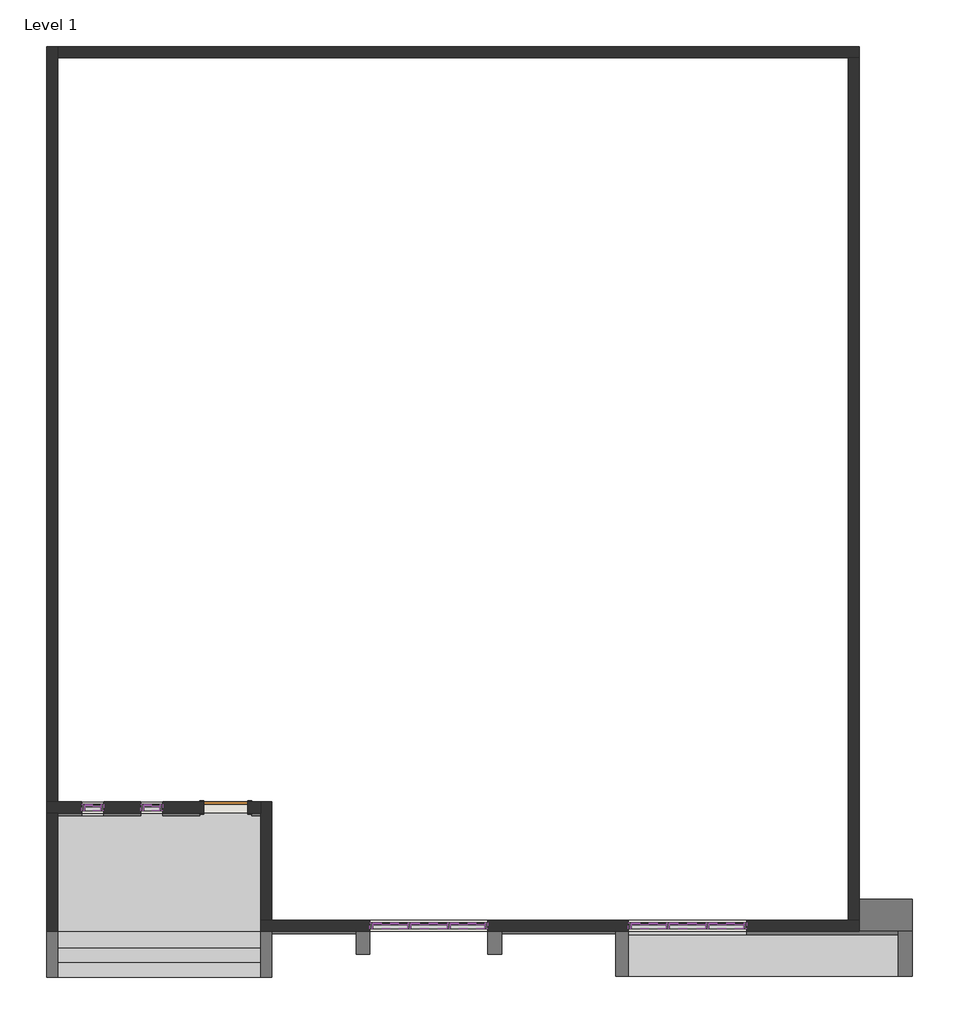
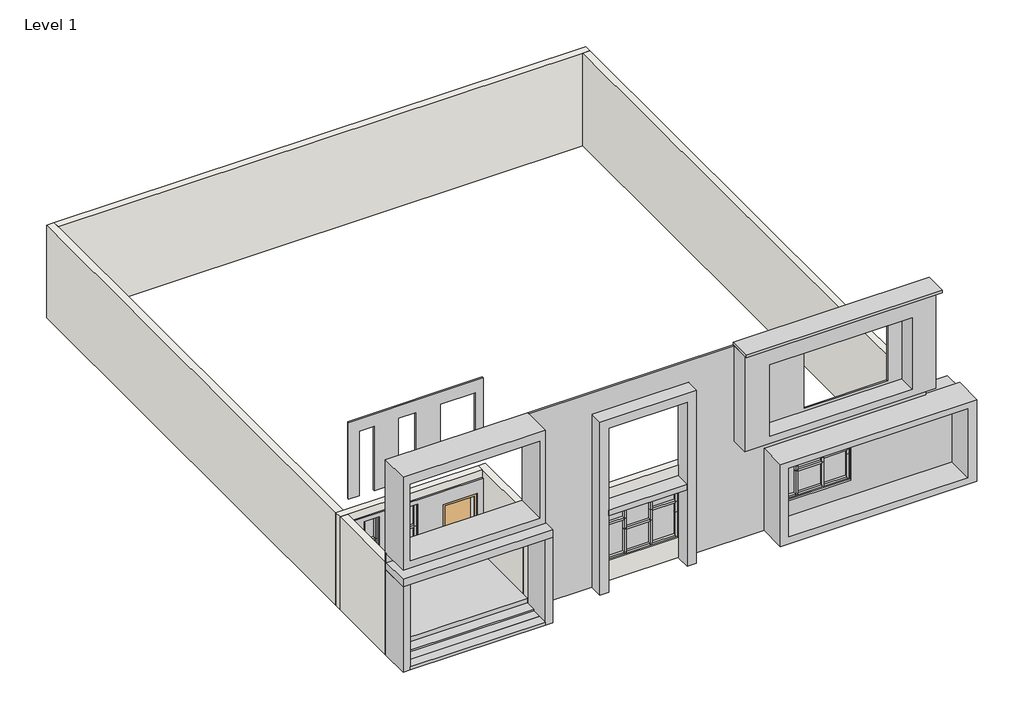
# One storey: 66 members, 18 plates, 7 walls, 3 proxies, 1 door.
"""IFC4 building model written with IfcOpenShell, lengths in millimetres."""

from ifc_helpers import new_model, si_unit, origin, origin_with_axes, place, context, project, spatial, polyline, outline, extrude, faceted_brep, transform, mapped, element, save
from components import generic_models_1_generic_models_1_0112e005, generic_models_2_generic_models_2_1d31d6de, generic_models_3_generic_models_3_58a4acd4, door_a90ba1ad, member_ff9f2d30, member_0c1408be, member_1407b1c2, member_43aa0f4e, member_63078a24, member_5ca2be8d, member_41a76b6e, member_7007ad49, member_abeaf8ac, member_aebd74a6, member_9d02be77, member_658e374b, member_8dafe1b6, member_798d6cad, member_876f8f00, member_3d7cb871, member_d7af48b5, member_00d00b53, member_8ca7f02a, member_f6f0dfdd, member_6e893292, member_cb8890cf, system_panel_glazed_59fe5a42, system_panel_glazed_f4e6dc7a, system_panel_glazed_28fed175, system_panel_glazed_9c7248e6, system_panel_glazed_f4f40b1b, system_panel_glazed_17d59646, system_panel_glazed_ecd9048c, system_panel_glazed_aaf6793b, system_panel_glazed_396e3693, system_panel_glazed_a956e29f, system_panel_glazed_64ba1ee3, system_panel_glazed_be4ca357, system_panel_glazed_edf5bdbe, system_panel_glazed_ddb2445b

model = new_model("IFC4")

# Units and contexts
model_context = context("Model", 3, world=origin())
ifc_project = project(units=[si_unit("LENGTHUNIT", "METRE", prefix="MILLI")], contexts=[model_context])

# Site, building, storey
site = spatial("IfcSite", under=ifc_project)
building = spatial("IfcBuilding", under=site)
storey = spatial("IfcBuildingStorey", under=building, Name="Level 1", Elevation=0.0)

# Proxies
placement = place(None, origin())
generic_models_1_generic_models_1_shape = generic_models_1_generic_models_1_0112e005(model_context)
element("IfcBuildingElementProxy", 1, Name="Generic Models 1 : Generic Models 1", ObjectType="Generic Models 1 : Generic Models 1", at=placement, inside=storey, context=model_context, shape_type="MappedRepresentation", body=[
    mapped(generic_models_1_generic_models_1_shape, transform((0.0, 0.0, 0.0), x_axis=(1.0, 0.0, 0.0), y_axis=(0.0, 1.0, 0.0), z_axis=(0.0, 0.0, 1.0))),
])
generic_models_2_generic_models_2_shape = generic_models_2_generic_models_2_1d31d6de(model_context)
element("IfcBuildingElementProxy", 2, Name="Generic Models 2 : Generic Models 2", ObjectType="Generic Models 2 : Generic Models 2", at=placement, inside=storey, context=model_context, shape_type="MappedRepresentation", body=[
    mapped(generic_models_2_generic_models_2_shape, transform((0.0, 0.0, 0.0), x_axis=(1.0, 0.0, 0.0), y_axis=(0.0, 1.0, 0.0), z_axis=(0.0, 0.0, 1.0))),
])
generic_models_3_generic_models_3_shape = generic_models_3_generic_models_3_58a4acd4(model_context)
element("IfcBuildingElementProxy", 3, Name="Generic Models 3 : Generic Models 3", ObjectType="Generic Models 3 : Generic Models 3", at=placement, inside=storey, context=model_context, shape_type="MappedRepresentation", body=[
    mapped(generic_models_3_generic_models_3_shape, transform((0.0, 0.0, 0.0), x_axis=(1.0, 0.0, 0.0), y_axis=(0.0, 1.0, 0.0), z_axis=(0.0, 0.0, 1.0))),
])

# Door
door_shape = door_a90ba1ad(model_context)
element("IfcDoor", 4, ObjectType="Single-Flush : 36\" x 84\"", at=placement, inside=storey, context=model_context, shape_type="MappedRepresentation", body=[
    mapped(door_shape, transform((685.139189, -10823.7602599, 152.4), x_axis=(-1.0, 0.0, 0.0), y_axis=(0.0, -1.0, 0.0), z_axis=(0.0, 0.0, 1.0))),
])

# Members
member_shape = member_ff9f2d30(model_context)
element("IfcMember", 5, ObjectType="Rectangular Mullion : 2.5\" x 5\" rectangular", at=placement, inside=storey, context=model_context, shape_type="MappedRepresentation", body=[
    mapped(member_shape, transform((-1892.960811, -10823.7602599, 2673.2296856), x_axis=(0.0, 0.0, 1.0), y_axis=(0.0, -1.0, 0.0), z_axis=(1.0, 0.0, 0.0))),
])
element("IfcMember", 6, ObjectType="Rectangular Mullion : 2.5\" x 5\" rectangular", at=placement, inside=storey, context=model_context, shape_type="MappedRepresentation", body=[
    mapped(member_shape, transform((-673.760811, -10823.7602599, 2663.3809799), x_axis=(0.0, 0.0, 1.0), y_axis=(0.0, -1.0, 0.0), z_axis=(1.0, 0.0, 0.0))),
])
element("IfcMember", 7, ObjectType="Rectangular Mullion : 2.5\" x 5\" rectangular", at=placement, inside=storey, context=model_context, shape_type="MappedRepresentation", body=[
    mapped(member_shape, transform((-2223.160811, -10823.7602599, 367.4911337), x_axis=(0.0, 0.0, -1.0), y_axis=(0.0, -1.0, 0.0), z_axis=(-1.0, 0.0, 0.0))),
])
element("IfcMember", 8, ObjectType="Rectangular Mullion : 2.5\" x 5\" rectangular", at=placement, inside=storey, context=model_context, shape_type="MappedRepresentation", body=[
    mapped(member_shape, transform((-1003.960811, -10823.7602599, 337.5681844), x_axis=(0.0, 0.0, -1.0), y_axis=(0.0, -1.0, 0.0), z_axis=(-1.0, 0.0, 0.0))),
])
member_2_shape = member_0c1408be(model_context)
element("IfcMember", 9, ObjectType="Rectangular Mullion : 2.5\" x 5\" rectangular", at=placement, inside=storey, context=model_context, shape_type="MappedRepresentation", body=[
    mapped(member_2_shape, transform((-1892.960811, -10823.7602599, 1136.070651), x_axis=(0.0, 0.0, 1.0), y_axis=(0.0, -1.0, 0.0), z_axis=(1.0, 0.0, 0.0))),
])
element("IfcMember", 10, ObjectType="Rectangular Mullion : 2.5\" x 5\" rectangular", at=placement, inside=storey, context=model_context, shape_type="MappedRepresentation", body=[
    mapped(member_2_shape, transform((-1892.960811, -10823.7602599, 1904.6501683), x_axis=(0.0, 0.0, 1.0), y_axis=(0.0, -1.0, 0.0), z_axis=(1.0, 0.0, 0.0))),
])
element("IfcMember", 11, ObjectType="Rectangular Mullion : 2.5\" x 5\" rectangular", at=placement, inside=storey, context=model_context, shape_type="MappedRepresentation", body=[
    mapped(member_2_shape, transform((-673.760811, -10823.7602599, 1888.1100481), x_axis=(0.0, 0.0, 1.0), y_axis=(0.0, -1.0, 0.0), z_axis=(1.0, 0.0, 0.0))),
])
element("IfcMember", 12, ObjectType="Rectangular Mullion : 2.5\" x 5\" rectangular", at=placement, inside=storey, context=model_context, shape_type="MappedRepresentation", body=[
    mapped(member_2_shape, transform((-673.760811, -10823.7602599, 1112.8391162), x_axis=(0.0, 0.0, 1.0), y_axis=(0.0, -1.0, 0.0), z_axis=(1.0, 0.0, 0.0))),
])
member_3_shape = member_1407b1c2(model_context)
element("IfcMember", 13, ObjectType="Rectangular Mullion : 2.5\" x 5\" rectangular", at=placement, inside=storey, context=model_context, shape_type="MappedRepresentation", body=[
    mapped(member_3_shape, transform((-2286.660811, -10823.7602599, 1136.070651), x_axis=(-1.0, 0.0, 0.0), y_axis=(0.0, -1.0, 0.0), z_axis=(0.0, 0.0, 1.0))),
])
element("IfcMember", 14, ObjectType="Rectangular Mullion : 2.5\" x 5\" rectangular", at=placement, inside=storey, context=model_context, shape_type="MappedRepresentation", body=[
    mapped(member_3_shape, transform((-1829.460811, -10823.7602599, 367.4911337), x_axis=(1.0, 0.0, 0.0), y_axis=(0.0, -1.0, 0.0), z_axis=(0.0, 0.0, -1.0))),
])
element("IfcMember", 15, ObjectType="Rectangular Mullion : 2.5\" x 5\" rectangular", at=placement, inside=storey, context=model_context, shape_type="MappedRepresentation", body=[
    mapped(member_3_shape, transform((-2286.660811, -10823.7602599, 1904.6501683), x_axis=(-1.0, 0.0, 0.0), y_axis=(0.0, -1.0, 0.0), z_axis=(0.0, 0.0, 1.0))),
])
element("IfcMember", 16, ObjectType="Rectangular Mullion : 2.5\" x 5\" rectangular", at=placement, inside=storey, context=model_context, shape_type="MappedRepresentation", body=[
    mapped(member_3_shape, transform((-2286.660811, -10823.7602599, 2673.2296856), x_axis=(-1.0, 0.0, 0.0), y_axis=(0.0, -1.0, 0.0), z_axis=(0.0, 0.0, 1.0))),
])
element("IfcMember", 17, ObjectType="Rectangular Mullion : 2.5\" x 5\" rectangular", at=placement, inside=storey, context=model_context, shape_type="MappedRepresentation", body=[
    mapped(member_3_shape, transform((-1829.460811, -10823.7602599, 1136.070651), x_axis=(1.0, 0.0, 0.0), y_axis=(0.0, -1.0, 0.0), z_axis=(0.0, 0.0, -1.0))),
])
element("IfcMember", 18, ObjectType="Rectangular Mullion : 2.5\" x 5\" rectangular", at=placement, inside=storey, context=model_context, shape_type="MappedRepresentation", body=[
    mapped(member_3_shape, transform((-1829.460811, -10823.7602599, 1904.6501683), x_axis=(1.0, 0.0, 0.0), y_axis=(0.0, -1.0, 0.0), z_axis=(0.0, 0.0, -1.0))),
])
member_4_shape = member_43aa0f4e(model_context)
element("IfcMember", 19, ObjectType="Rectangular Mullion : 2.5\" x 5\" rectangular", at=placement, inside=storey, context=model_context, shape_type="MappedRepresentation", body=[
    mapped(member_4_shape, transform((-1067.460811, -10823.7602599, 2663.3809799), x_axis=(-1.0, 0.0, 0.0), y_axis=(0.0, -1.0, 0.0), z_axis=(0.0, 0.0, 1.0))),
])
element("IfcMember", 20, ObjectType="Rectangular Mullion : 2.5\" x 5\" rectangular", at=placement, inside=storey, context=model_context, shape_type="MappedRepresentation", body=[
    mapped(member_4_shape, transform((-610.260811, -10823.7602599, 1888.1100481), x_axis=(1.0, 0.0, 0.0), y_axis=(0.0, -1.0, 0.0), z_axis=(0.0, 0.0, -1.0))),
])
element("IfcMember", 21, ObjectType="Rectangular Mullion : 2.5\" x 5\" rectangular", at=placement, inside=storey, context=model_context, shape_type="MappedRepresentation", body=[
    mapped(member_4_shape, transform((-1067.460811, -10823.7602599, 1888.1100481), x_axis=(-1.0, 0.0, 0.0), y_axis=(0.0, -1.0, 0.0), z_axis=(0.0, 0.0, 1.0))),
])
element("IfcMember", 22, ObjectType="Rectangular Mullion : 2.5\" x 5\" rectangular", at=placement, inside=storey, context=model_context, shape_type="MappedRepresentation", body=[
    mapped(member_4_shape, transform((-610.260811, -10823.7602599, 1112.8391162), x_axis=(1.0, 0.0, 0.0), y_axis=(0.0, -1.0, 0.0), z_axis=(0.0, 0.0, -1.0))),
])
element("IfcMember", 23, ObjectType="Rectangular Mullion : 2.5\" x 5\" rectangular", at=placement, inside=storey, context=model_context, shape_type="MappedRepresentation", body=[
    mapped(member_4_shape, transform((-1067.460811, -10823.7602599, 1112.8391162), x_axis=(-1.0, 0.0, 0.0), y_axis=(0.0, -1.0, 0.0), z_axis=(0.0, 0.0, 1.0))),
])
element("IfcMember", 24, ObjectType="Rectangular Mullion : 2.5\" x 5\" rectangular", at=placement, inside=storey, context=model_context, shape_type="MappedRepresentation", body=[
    mapped(member_4_shape, transform((-610.260811, -10823.7602599, 337.5681844), x_axis=(1.0, 0.0, 0.0), y_axis=(0.0, -1.0, 0.0), z_axis=(0.0, 0.0, -1.0))),
])
member_5_shape = member_63078a24(model_context)
element("IfcMember", 25, ObjectType="Rectangular Mullion : 2.5\" x 5\" rectangular", at=placement, inside=storey, context=model_context, shape_type="MappedRepresentation", body=[
    mapped(member_5_shape, transform((3656.939189, -13262.1602599, 1486.3026682), x_axis=(-1.0, 0.0, 0.0), y_axis=(0.0, -1.0, 0.0), z_axis=(0.0, 0.0, 1.0))),
])
member_6_shape = member_5ca2be8d(model_context)
element("IfcMember", 26, ObjectType="Rectangular Mullion : 2.5\" x 5\" rectangular", at=placement, inside=storey, context=model_context, shape_type="MappedRepresentation", body=[
    mapped(member_6_shape, transform((3656.939189, -13262.1602599, 1828.1310444), x_axis=(-1.0, 0.0, 0.0), y_axis=(0.0, -1.0, 0.0), z_axis=(0.0, 0.0, 1.0))),
])
member_7_shape = member_41a76b6e(model_context)
element("IfcMember", 27, ObjectType="Rectangular Mullion : 2.5\" x 5\" rectangular", at=placement, inside=storey, context=model_context, shape_type="MappedRepresentation", body=[
    mapped(member_7_shape, transform((3656.939189, -13262.1602599, 2511.7877969), x_axis=(-1.0, 0.0, 0.0), y_axis=(0.0, -1.0, 0.0), z_axis=(0.0, 0.0, 1.0))),
])
member_8_shape = member_7007ad49(model_context)
element("IfcMember", 28, ObjectType="Rectangular Mullion : 2.5\" x 5\" rectangular", at=placement, inside=storey, context=model_context, shape_type="MappedRepresentation", body=[
    mapped(member_8_shape, transform((4437.989189, -13262.1602599, 2511.7877969), x_axis=(0.0, 0.0, 1.0), y_axis=(0.0, -1.0, 0.0), z_axis=(1.0, 0.0, 0.0))),
])
element("IfcMember", 29, ObjectType="Rectangular Mullion : 2.5\" x 5\" rectangular", at=placement, inside=storey, context=model_context, shape_type="MappedRepresentation", body=[
    mapped(member_8_shape, transform((6031.839189, -13262.1602599, 2511.7877969), x_axis=(0.0, 0.0, 1.0), y_axis=(0.0, -1.0, 0.0), z_axis=(1.0, 0.0, 0.0))),
])
element("IfcMember", 30, ObjectType="Rectangular Mullion : 2.5\" x 5\" rectangular", at=placement, inside=storey, context=model_context, shape_type="MappedRepresentation", body=[
    mapped(member_8_shape, transform((9771.989189, -13262.1602599, 2489.531124), x_axis=(0.0, 0.0, 1.0), y_axis=(0.0, -1.0, 0.0), z_axis=(1.0, 0.0, 0.0))),
])
element("IfcMember", 31, ObjectType="Rectangular Mullion : 2.5\" x 5\" rectangular", at=placement, inside=storey, context=model_context, shape_type="MappedRepresentation", body=[
    mapped(member_8_shape, transform((11365.839189, -13262.1602599, 2489.531124), x_axis=(0.0, 0.0, 1.0), y_axis=(0.0, -1.0, 0.0), z_axis=(1.0, 0.0, 0.0))),
])
element("IfcMember", 32, ObjectType="Rectangular Mullion : 2.5\" x 5\" rectangular", at=placement, inside=storey, context=model_context, shape_type="MappedRepresentation", body=[
    mapped(member_8_shape, transform((5314.289189, -13262.1602599, 665.9145653), x_axis=(0.0, 0.0, -1.0), y_axis=(0.0, -1.0, 0.0), z_axis=(-1.0, 0.0, 0.0))),
])
element("IfcMember", 33, ObjectType="Rectangular Mullion : 2.5\" x 5\" rectangular", at=placement, inside=storey, context=model_context, shape_type="MappedRepresentation", body=[
    mapped(member_8_shape, transform((3720.439189, -13262.1602599, 665.9145653), x_axis=(0.0, 0.0, -1.0), y_axis=(0.0, -1.0, 0.0), z_axis=(-1.0, 0.0, 0.0))),
])
element("IfcMember", 34, ObjectType="Rectangular Mullion : 2.5\" x 5\" rectangular", at=placement, inside=storey, context=model_context, shape_type="MappedRepresentation", body=[
    mapped(member_8_shape, transform((10648.289189, -13262.1602599, 718.1429127), x_axis=(0.0, 0.0, -1.0), y_axis=(0.0, -1.0, 0.0), z_axis=(-1.0, 0.0, 0.0))),
])
element("IfcMember", 35, ObjectType="Rectangular Mullion : 2.5\" x 5\" rectangular", at=placement, inside=storey, context=model_context, shape_type="MappedRepresentation", body=[
    mapped(member_8_shape, transform((9054.439189, -13262.1602599, 718.1429127), x_axis=(0.0, 0.0, -1.0), y_axis=(0.0, -1.0, 0.0), z_axis=(-1.0, 0.0, 0.0))),
])
member_9_shape = member_abeaf8ac(model_context)
element("IfcMember", 36, ObjectType="Rectangular Mullion : 2.5\" x 5\" rectangular", at=placement, inside=storey, context=model_context, shape_type="MappedRepresentation", body=[
    mapped(member_9_shape, transform((6031.839189, -13262.1602599, 1828.1310444), x_axis=(0.0, 0.0, 1.0), y_axis=(0.0, -1.0, 0.0), z_axis=(1.0, 0.0, 0.0))),
])
element("IfcMember", 37, ObjectType="Rectangular Mullion : 2.5\" x 5\" rectangular", at=placement, inside=storey, context=model_context, shape_type="MappedRepresentation", body=[
    mapped(member_9_shape, transform((4437.989189, -13262.1602599, 1828.1310444), x_axis=(0.0, 0.0, 1.0), y_axis=(0.0, -1.0, 0.0), z_axis=(1.0, 0.0, 0.0))),
])
element("IfcMember", 38, ObjectType="Rectangular Mullion : 2.5\" x 5\" rectangular", at=placement, inside=storey, context=model_context, shape_type="MappedRepresentation", body=[
    mapped(member_9_shape, transform((9771.989189, -13262.1602599, 1752.931124), x_axis=(0.0, 0.0, 1.0), y_axis=(0.0, -1.0, 0.0), z_axis=(1.0, 0.0, 0.0))),
])
element("IfcMember", 39, ObjectType="Rectangular Mullion : 2.5\" x 5\" rectangular", at=placement, inside=storey, context=model_context, shape_type="MappedRepresentation", body=[
    mapped(member_9_shape, transform((11365.839189, -13262.1602599, 1676.731124), x_axis=(0.0, 0.0, 1.0), y_axis=(0.0, -1.0, 0.0), z_axis=(1.0, 0.0, 0.0))),
])
member_10_shape = member_aebd74a6(model_context)
element("IfcMember", 40, ObjectType="Rectangular Mullion : 2.5\" x 5\" rectangular", at=placement, inside=storey, context=model_context, shape_type="MappedRepresentation", body=[
    mapped(member_10_shape, transform((4469.739189, -13262.1602599, 1828.1310444), x_axis=(1.0, 0.0, 0.0), y_axis=(0.0, -1.0, 0.0), z_axis=(0.0, 0.0, -1.0))),
])
element("IfcMember", 41, ObjectType="Rectangular Mullion : 2.5\" x 5\" rectangular", at=placement, inside=storey, context=model_context, shape_type="MappedRepresentation", body=[
    mapped(member_10_shape, transform((5282.539189, -13262.1602599, 1828.1310444), x_axis=(1.0, 0.0, 0.0), y_axis=(0.0, -1.0, 0.0), z_axis=(0.0, 0.0, -1.0))),
])
member_11_shape = member_9d02be77(model_context)
element("IfcMember", 42, ObjectType="Rectangular Mullion : 2.5\" x 5\" rectangular", at=placement, inside=storey, context=model_context, shape_type="MappedRepresentation", body=[
    mapped(member_11_shape, transform((5250.789189, -13262.1602599, 2511.7877969), x_axis=(0.0, 0.0, 1.0), y_axis=(0.0, -1.0, 0.0), z_axis=(1.0, 0.0, 0.0))),
])
element("IfcMember", 43, ObjectType="Rectangular Mullion : 2.5\" x 5\" rectangular", at=placement, inside=storey, context=model_context, shape_type="MappedRepresentation", body=[
    mapped(member_11_shape, transform((10584.789189, -13262.1602599, 2489.531124), x_axis=(0.0, 0.0, 1.0), y_axis=(0.0, -1.0, 0.0), z_axis=(1.0, 0.0, 0.0))),
])
element("IfcMember", 44, ObjectType="Rectangular Mullion : 2.5\" x 5\" rectangular", at=placement, inside=storey, context=model_context, shape_type="MappedRepresentation", body=[
    mapped(member_11_shape, transform((4501.489189, -13262.1602599, 665.9145653), x_axis=(0.0, 0.0, -1.0), y_axis=(0.0, -1.0, 0.0), z_axis=(-1.0, 0.0, 0.0))),
])
element("IfcMember", 45, ObjectType="Rectangular Mullion : 2.5\" x 5\" rectangular", at=placement, inside=storey, context=model_context, shape_type="MappedRepresentation", body=[
    mapped(member_11_shape, transform((9835.489189, -13262.1602599, 718.1429127), x_axis=(0.0, 0.0, -1.0), y_axis=(0.0, -1.0, 0.0), z_axis=(-1.0, 0.0, 0.0))),
])
member_12_shape = member_658e374b(model_context)
element("IfcMember", 46, ObjectType="Rectangular Mullion : 2.5\" x 5\" rectangular", at=placement, inside=storey, context=model_context, shape_type="MappedRepresentation", body=[
    mapped(member_12_shape, transform((4469.739189, -13262.1602599, 1486.3026682), x_axis=(1.0, 0.0, 0.0), y_axis=(0.0, -1.0, 0.0), z_axis=(0.0, 0.0, -1.0))),
])
element("IfcMember", 47, ObjectType="Rectangular Mullion : 2.5\" x 5\" rectangular", at=placement, inside=storey, context=model_context, shape_type="MappedRepresentation", body=[
    mapped(member_12_shape, transform((5282.539189, -13262.1602599, 1486.3026682), x_axis=(1.0, 0.0, 0.0), y_axis=(0.0, -1.0, 0.0), z_axis=(0.0, 0.0, -1.0))),
])
member_13_shape = member_8dafe1b6(model_context)
element("IfcMember", 48, ObjectType="Rectangular Mullion : 2.5\" x 5\" rectangular", at=placement, inside=storey, context=model_context, shape_type="MappedRepresentation", body=[
    mapped(member_13_shape, transform((4469.739189, -13262.1602599, 665.9145653), x_axis=(1.0, 0.0, 0.0), y_axis=(0.0, -1.0, 0.0), z_axis=(0.0, 0.0, -1.0))),
])
element("IfcMember", 49, ObjectType="Rectangular Mullion : 2.5\" x 5\" rectangular", at=placement, inside=storey, context=model_context, shape_type="MappedRepresentation", body=[
    mapped(member_13_shape, transform((5282.539189, -13262.1602599, 665.9145653), x_axis=(1.0, 0.0, 0.0), y_axis=(0.0, -1.0, 0.0), z_axis=(0.0, 0.0, -1.0))),
])
member_14_shape = member_798d6cad(model_context)
element("IfcMember", 50, ObjectType="Rectangular Mullion : 2.5\" x 5\" rectangular", at=placement, inside=storey, context=model_context, shape_type="MappedRepresentation", body=[
    mapped(member_14_shape, transform((5250.789189, -13262.1602599, 1486.3026682), x_axis=(0.0, 0.0, 1.0), y_axis=(0.0, -1.0, 0.0), z_axis=(1.0, 0.0, 0.0))),
])
element("IfcMember", 51, ObjectType="Rectangular Mullion : 2.5\" x 5\" rectangular", at=placement, inside=storey, context=model_context, shape_type="MappedRepresentation", body=[
    mapped(member_14_shape, transform((10584.789189, -13262.1602599, 1524.331124), x_axis=(0.0, 0.0, 1.0), y_axis=(0.0, -1.0, 0.0), z_axis=(1.0, 0.0, 0.0))),
])
element("IfcMember", 52, ObjectType="Rectangular Mullion : 2.5\" x 5\" rectangular", at=placement, inside=storey, context=model_context, shape_type="MappedRepresentation", body=[
    mapped(member_7_shape, transform((6095.339189, -13262.1602599, 1828.1310444), x_axis=(1.0, 0.0, 0.0), y_axis=(0.0, -1.0, 0.0), z_axis=(0.0, 0.0, -1.0))),
])
element("IfcMember", 53, ObjectType="Rectangular Mullion : 2.5\" x 5\" rectangular", at=placement, inside=storey, context=model_context, shape_type="MappedRepresentation", body=[
    mapped(member_6_shape, transform((6095.339189, -13262.1602599, 1486.3026682), x_axis=(1.0, 0.0, 0.0), y_axis=(0.0, -1.0, 0.0), z_axis=(0.0, 0.0, -1.0))),
])
element("IfcMember", 54, ObjectType="Rectangular Mullion : 2.5\" x 5\" rectangular", at=placement, inside=storey, context=model_context, shape_type="MappedRepresentation", body=[
    mapped(member_5_shape, transform((6095.339189, -13262.1602599, 665.9145653), x_axis=(1.0, 0.0, 0.0), y_axis=(0.0, -1.0, 0.0), z_axis=(0.0, 0.0, -1.0))),
])
member_15_shape = member_876f8f00(model_context)
element("IfcMember", 55, ObjectType="Rectangular Mullion : 2.5\" x 5\" rectangular", at=placement, inside=storey, context=model_context, shape_type="MappedRepresentation", body=[
    mapped(member_15_shape, transform((8990.939189, -13262.1602599, 1676.731124), x_axis=(-1.0, 0.0, 0.0), y_axis=(0.0, -1.0, 0.0), z_axis=(0.0, 0.0, 1.0))),
])
member_16_shape = member_3d7cb871(model_context)
element("IfcMember", 56, ObjectType="Rectangular Mullion : 2.5\" x 5\" rectangular", at=placement, inside=storey, context=model_context, shape_type="MappedRepresentation", body=[
    mapped(member_16_shape, transform((8990.939189, -13262.1602599, 1752.931124), x_axis=(-1.0, 0.0, 0.0), y_axis=(0.0, -1.0, 0.0), z_axis=(0.0, 0.0, 1.0))),
])
member_17_shape = member_d7af48b5(model_context)
element("IfcMember", 57, ObjectType="Rectangular Mullion : 2.5\" x 5\" rectangular", at=placement, inside=storey, context=model_context, shape_type="MappedRepresentation", body=[
    mapped(member_17_shape, transform((8990.939189, -13262.1602599, 2489.531124), x_axis=(-1.0, 0.0, 0.0), y_axis=(0.0, -1.0, 0.0), z_axis=(0.0, 0.0, 1.0))),
])
member_18_shape = member_00d00b53(model_context)
element("IfcMember", 58, ObjectType="Rectangular Mullion : 2.5\" x 5\" rectangular", at=placement, inside=storey, context=model_context, shape_type="MappedRepresentation", body=[
    mapped(member_18_shape, transform((9803.739189, -13262.1602599, 1676.731124), x_axis=(1.0, 0.0, 0.0), y_axis=(0.0, -1.0, 0.0), z_axis=(0.0, 0.0, -1.0))),
])
member_19_shape = member_8ca7f02a(model_context)
element("IfcMember", 59, ObjectType="Rectangular Mullion : 2.5\" x 5\" rectangular", at=placement, inside=storey, context=model_context, shape_type="MappedRepresentation", body=[
    mapped(member_19_shape, transform((9803.739189, -13262.1602599, 1752.931124), x_axis=(1.0, 0.0, 0.0), y_axis=(0.0, -1.0, 0.0), z_axis=(0.0, 0.0, -1.0))),
])
member_20_shape = member_f6f0dfdd(model_context)
element("IfcMember", 60, ObjectType="Rectangular Mullion : 2.5\" x 5\" rectangular", at=placement, inside=storey, context=model_context, shape_type="MappedRepresentation", body=[
    mapped(member_20_shape, transform((9803.739189, -13262.1602599, 1524.331124), x_axis=(1.0, 0.0, 0.0), y_axis=(0.0, -1.0, 0.0), z_axis=(0.0, 0.0, -1.0))),
])
element("IfcMember", 61, ObjectType="Rectangular Mullion : 2.5\" x 5\" rectangular", at=placement, inside=storey, context=model_context, shape_type="MappedRepresentation", body=[
    mapped(member_19_shape, transform((10616.539189, -13262.1602599, 1752.931124), x_axis=(1.0, 0.0, 0.0), y_axis=(0.0, -1.0, 0.0), z_axis=(0.0, 0.0, -1.0))),
])
element("IfcMember", 62, ObjectType="Rectangular Mullion : 2.5\" x 5\" rectangular", at=placement, inside=storey, context=model_context, shape_type="MappedRepresentation", body=[
    mapped(member_20_shape, transform((10616.539189, -13262.1602599, 1524.331124), x_axis=(1.0, 0.0, 0.0), y_axis=(0.0, -1.0, 0.0), z_axis=(0.0, 0.0, -1.0))),
])
element("IfcMember", 63, ObjectType="Rectangular Mullion : 2.5\" x 5\" rectangular", at=placement, inside=storey, context=model_context, shape_type="MappedRepresentation", body=[
    mapped(member_18_shape, transform((10616.539189, -13262.1602599, 1676.731124), x_axis=(1.0, 0.0, 0.0), y_axis=(0.0, -1.0, 0.0), z_axis=(0.0, 0.0, -1.0))),
])
element("IfcMember", 64, ObjectType="Rectangular Mullion : 2.5\" x 5\" rectangular", at=placement, inside=storey, context=model_context, shape_type="MappedRepresentation", body=[
    mapped(member_15_shape, transform((11429.339189, -13262.1602599, 1524.331124), x_axis=(1.0, 0.0, 0.0), y_axis=(0.0, -1.0, 0.0), z_axis=(0.0, 0.0, -1.0))),
])
element("IfcMember", 65, ObjectType="Rectangular Mullion : 2.5\" x 5\" rectangular", at=placement, inside=storey, context=model_context, shape_type="MappedRepresentation", body=[
    mapped(member_16_shape, transform((11429.339189, -13262.1602599, 1676.731124), x_axis=(1.0, 0.0, 0.0), y_axis=(0.0, -1.0, 0.0), z_axis=(0.0, 0.0, -1.0))),
])
element("IfcMember", 66, ObjectType="Rectangular Mullion : 2.5\" x 5\" rectangular", at=placement, inside=storey, context=model_context, shape_type="MappedRepresentation", body=[
    mapped(member_17_shape, transform((11429.339189, -13262.1602599, 1752.931124), x_axis=(1.0, 0.0, 0.0), y_axis=(0.0, -1.0, 0.0), z_axis=(0.0, 0.0, -1.0))),
])
member_21_shape = member_6e893292(model_context)
element("IfcMember", 67, ObjectType="Rectangular Mullion : 2.5\" x 5\" rectangular", at=placement, inside=storey, context=model_context, shape_type="MappedRepresentation", body=[
    mapped(member_21_shape, transform((9803.739189, -13262.1602599, 718.1429127), x_axis=(1.0, 0.0, 0.0), y_axis=(0.0, -1.0, 0.0), z_axis=(0.0, 0.0, -1.0))),
])
element("IfcMember", 68, ObjectType="Rectangular Mullion : 2.5\" x 5\" rectangular", at=placement, inside=storey, context=model_context, shape_type="MappedRepresentation", body=[
    mapped(member_21_shape, transform((10616.539189, -13262.1602599, 718.1429127), x_axis=(1.0, 0.0, 0.0), y_axis=(0.0, -1.0, 0.0), z_axis=(0.0, 0.0, -1.0))),
])
member_22_shape = member_cb8890cf(model_context)
element("IfcMember", 69, ObjectType="Rectangular Mullion : 2.5\" x 5\" rectangular", at=placement, inside=storey, context=model_context, shape_type="MappedRepresentation", body=[
    mapped(member_22_shape, transform((8990.939189, -13262.1602599, 1524.331124), x_axis=(-1.0, 0.0, 0.0), y_axis=(0.0, -1.0, 0.0), z_axis=(0.0, 0.0, 1.0))),
])
element("IfcMember", 70, ObjectType="Rectangular Mullion : 2.5\" x 5\" rectangular", at=placement, inside=storey, context=model_context, shape_type="MappedRepresentation", body=[
    mapped(member_22_shape, transform((11429.339189, -13262.1602599, 718.1429127), x_axis=(1.0, 0.0, 0.0), y_axis=(0.0, -1.0, 0.0), z_axis=(0.0, 0.0, -1.0))),
])

# Plates
system_panel_glazed_shape = system_panel_glazed_59fe5a42(model_context)
element("IfcPlate", 71, ObjectType="System Panel : Glazed", at=placement, inside=storey, context=model_context, shape_type="MappedRepresentation", body=[
    mapped(system_panel_glazed_shape, transform((-2058.060811, -10823.7602599, 1167.820651), x_axis=(1.0, 0.0, 0.0), y_axis=(0.0, 1.0, 0.0), z_axis=(0.0, 0.0, 1.0))),
])
system_panel_glazed_2_shape = system_panel_glazed_f4e6dc7a(model_context)
element("IfcPlate", 72, ObjectType="System Panel : Glazed", at=placement, inside=storey, context=model_context, shape_type="MappedRepresentation", body=[
    mapped(system_panel_glazed_2_shape, transform((-2058.060811, -10823.7602599, 430.9911337), x_axis=(1.0, 0.0, 0.0), y_axis=(0.0, 1.0, 0.0), z_axis=(0.0, 0.0, 1.0))),
])
element("IfcPlate", 73, ObjectType="System Panel : Glazed", at=placement, inside=storey, context=model_context, shape_type="MappedRepresentation", body=[
    mapped(system_panel_glazed_2_shape, transform((-2058.060811, -10823.7602599, 1936.4001683), x_axis=(1.0, 0.0, 0.0), y_axis=(0.0, 1.0, 0.0), z_axis=(0.0, 0.0, 1.0))),
])
system_panel_glazed_3_shape = system_panel_glazed_28fed175(model_context)
element("IfcPlate", 74, ObjectType="System Panel : Glazed", at=placement, inside=storey, context=model_context, shape_type="MappedRepresentation", body=[
    mapped(system_panel_glazed_3_shape, transform((-838.860811, -10823.7602599, 401.0681844), x_axis=(1.0, 0.0, 0.0), y_axis=(0.0, 1.0, 0.0), z_axis=(0.0, 0.0, 1.0))),
])
element("IfcPlate", 75, ObjectType="System Panel : Glazed", at=placement, inside=storey, context=model_context, shape_type="MappedRepresentation", body=[
    mapped(system_panel_glazed_3_shape, transform((-838.860811, -10823.7602599, 1919.8600481), x_axis=(1.0, 0.0, 0.0), y_axis=(0.0, 1.0, 0.0), z_axis=(0.0, 0.0, 1.0))),
])
system_panel_glazed_4_shape = system_panel_glazed_9c7248e6(model_context)
element("IfcPlate", 76, ObjectType="System Panel : Glazed", at=placement, inside=storey, context=model_context, shape_type="MappedRepresentation", body=[
    mapped(system_panel_glazed_4_shape, transform((-838.860811, -10823.7602599, 1144.5891162), x_axis=(1.0, 0.0, 0.0), y_axis=(0.0, 1.0, 0.0), z_axis=(0.0, 0.0, 1.0))),
])
system_panel_glazed_5_shape = system_panel_glazed_f4f40b1b(model_context)
element("IfcPlate", 77, ObjectType="System Panel : Glazed", at=placement, inside=storey, context=model_context, shape_type="MappedRepresentation", body=[
    mapped(system_panel_glazed_5_shape, transform((4079.214189, -13262.1602599, 729.4145653), x_axis=(1.0, 0.0, 0.0), y_axis=(0.0, 1.0, 0.0), z_axis=(0.0, 0.0, 1.0))),
])
element("IfcPlate", 78, ObjectType="System Panel : Glazed", at=placement, inside=storey, context=model_context, shape_type="MappedRepresentation", body=[
    mapped(system_panel_glazed_5_shape, transform((5673.064189, -13262.1602599, 729.4145653), x_axis=(1.0, 0.0, 0.0), y_axis=(0.0, 1.0, 0.0), z_axis=(0.0, 0.0, 1.0))),
])
system_panel_glazed_6_shape = system_panel_glazed_17d59646(model_context)
element("IfcPlate", 79, ObjectType="System Panel : Glazed", at=placement, inside=storey, context=model_context, shape_type="MappedRepresentation", body=[
    mapped(system_panel_glazed_6_shape, transform((4079.214189, -13262.1602599, 1859.8810444), x_axis=(1.0, 0.0, 0.0), y_axis=(0.0, 1.0, 0.0), z_axis=(0.0, 0.0, 1.0))),
])
element("IfcPlate", 80, ObjectType="System Panel : Glazed", at=placement, inside=storey, context=model_context, shape_type="MappedRepresentation", body=[
    mapped(system_panel_glazed_6_shape, transform((5673.064189, -13262.1602599, 1859.8810444), x_axis=(1.0, 0.0, 0.0), y_axis=(0.0, 1.0, 0.0), z_axis=(0.0, 0.0, 1.0))),
])
system_panel_glazed_7_shape = system_panel_glazed_ecd9048c(model_context)
element("IfcPlate", 81, ObjectType="System Panel : Glazed", at=placement, inside=storey, context=model_context, shape_type="MappedRepresentation", body=[
    mapped(system_panel_glazed_7_shape, transform((4876.139189, -13262.1602599, 729.4145653), x_axis=(1.0, 0.0, 0.0), y_axis=(0.0, 1.0, 0.0), z_axis=(0.0, 0.0, 1.0))),
])
system_panel_glazed_8_shape = system_panel_glazed_aaf6793b(model_context)
element("IfcPlate", 82, ObjectType="System Panel : Glazed", at=placement, inside=storey, context=model_context, shape_type="MappedRepresentation", body=[
    mapped(system_panel_glazed_8_shape, transform((4876.139189, -13262.1602599, 1518.0526682), x_axis=(1.0, 0.0, 0.0), y_axis=(0.0, 1.0, 0.0), z_axis=(0.0, 0.0, 1.0))),
])
system_panel_glazed_9_shape = system_panel_glazed_396e3693(model_context)
element("IfcPlate", 83, ObjectType="System Panel : Glazed", at=placement, inside=storey, context=model_context, shape_type="MappedRepresentation", body=[
    mapped(system_panel_glazed_9_shape, transform((9413.214189, -13262.1602599, 1784.681124), x_axis=(1.0, 0.0, 0.0), y_axis=(0.0, 1.0, 0.0), z_axis=(0.0, 0.0, 1.0))),
])
system_panel_glazed_10_shape = system_panel_glazed_a956e29f(model_context)
element("IfcPlate", 84, ObjectType="System Panel : Glazed", at=placement, inside=storey, context=model_context, shape_type="MappedRepresentation", body=[
    mapped(system_panel_glazed_10_shape, transform((10210.139189, -13262.1602599, 1556.081124), x_axis=(1.0, 0.0, 0.0), y_axis=(0.0, 1.0, 0.0), z_axis=(0.0, 0.0, 1.0))),
])
system_panel_glazed_11_shape = system_panel_glazed_64ba1ee3(model_context)
element("IfcPlate", 85, ObjectType="System Panel : Glazed", at=placement, inside=storey, context=model_context, shape_type="MappedRepresentation", body=[
    mapped(system_panel_glazed_11_shape, transform((11007.064189, -13262.1602599, 1708.481124), x_axis=(1.0, 0.0, 0.0), y_axis=(0.0, 1.0, 0.0), z_axis=(0.0, 0.0, 1.0))),
])
system_panel_glazed_12_shape = system_panel_glazed_be4ca357(model_context)
element("IfcPlate", 86, ObjectType="System Panel : Glazed", at=placement, inside=storey, context=model_context, shape_type="MappedRepresentation", body=[
    mapped(system_panel_glazed_12_shape, transform((9413.214189, -13262.1602599, 781.6429127), x_axis=(1.0, 0.0, 0.0), y_axis=(0.0, 1.0, 0.0), z_axis=(0.0, 0.0, 1.0))),
])
system_panel_glazed_13_shape = system_panel_glazed_edf5bdbe(model_context)
element("IfcPlate", 87, ObjectType="System Panel : Glazed", at=placement, inside=storey, context=model_context, shape_type="MappedRepresentation", body=[
    mapped(system_panel_glazed_13_shape, transform((10210.139189, -13262.1602599, 781.6429127), x_axis=(1.0, 0.0, 0.0), y_axis=(0.0, 1.0, 0.0), z_axis=(0.0, 0.0, 1.0))),
])
system_panel_glazed_14_shape = system_panel_glazed_ddb2445b(model_context)
element("IfcPlate", 88, ObjectType="System Panel : Glazed", at=placement, inside=storey, context=model_context, shape_type="MappedRepresentation", body=[
    mapped(system_panel_glazed_14_shape, transform((11007.064189, -13262.1602599, 781.6429127), x_axis=(1.0, 0.0, 0.0), y_axis=(0.0, 1.0, 0.0), z_axis=(0.0, 0.0, 1.0))),
])

# Walls
element("IfcWall", 89, ObjectType="9\"", at=placement, inside=storey, context=model_context, shape_type="Brep", body=[
    faceted_brep([(13753.439189, -13147.8602599, 0.0), (13524.839189, -13147.8602599, 0.0), (1637.639189, -13147.8602599, 0.0), (1409.039189, -13147.8602599, 0.0), (1409.039189, -13147.8602599, 3048.0), (1637.639189, -13147.8602599, 3048.0), (13524.839189, -13147.8602599, 3048.0), (13753.439189, -13147.8602599, 3048.0), (3656.939189, -13147.8602599, 2511.7877969), (3656.939189, -13147.8602599, 665.9145653), (6095.339189, -13147.8602599, 665.9145653), (6095.339189, -13147.8602599, 2511.7877969), (8990.939189, -13147.8602599, 2489.531124), (8990.939189, -13147.8602599, 718.1429127), (11429.339189, -13147.8602599, 718.1429127), (11429.339189, -13147.8602599, 2489.531124), (1409.039189, -13376.4602599, 0.0), (13753.439189, -13376.4602599, 0.0), (13753.439189, -13376.4602599, 3048.0), (1409.039189, -13376.4602599, 3048.0), (3656.939189, -13376.4602599, 665.9145653), (3656.939189, -13376.4602599, 2511.7877969), (6095.339189, -13376.4602599, 2511.7877969), (6095.339189, -13376.4602599, 665.9145653), (8990.939189, -13376.4602599, 718.1429127), (8990.939189, -13376.4602599, 2489.531124), (11429.339189, -13376.4602599, 2489.531124), (11429.339189, -13376.4602599, 718.1429127)], [[[0, 1, 2, 3, 4, 5, 6, 7], [8, 9, 10, 11], [12, 13, 14, 15]], [[16, 17, 18, 19], [20, 21, 22, 23], [24, 25, 26, 27]], [[4, 3, 16, 19]], [[0, 7, 18, 17]], [[8, 21, 20, 9]], [[21, 8, 11, 22]], [[22, 11, 10, 23]], [[9, 20, 23, 10]], [[24, 13, 12, 25]], [[25, 12, 15, 26]], [[26, 15, 14, 27]], [[13, 24, 27, 14]], [[3, 2, 1, 0, 17, 16]], [[7, 6, 5, 4, 19, 18]]]),
])
element("IfcWall", 90, ObjectType="9\"", at=placement, inside=storey, context=model_context, shape_type="Brep", body=[
    faceted_brep([(1637.639189, -13147.8602599, 0.0), (1637.639189, -10709.4602599, 0.0), (1637.639189, -10709.4602599, 3048.0), (1637.639189, -13147.8602599, 3048.0), (1409.039189, -13147.8602599, 0.0), (1409.039189, -13147.8602599, 3048.0), (1409.039189, -10938.0602599, 3048.0), (1409.039189, -10709.4602599, 3048.0), (1409.039189, -10709.4602599, 0.0), (1409.039189, -10938.0602599, 0.0)], [[[0, 1, 2, 3]], [[4, 5, 6, 7, 8, 9]], [[1, 0, 4, 9, 8]], [[3, 2, 7, 6, 5]], [[0, 3, 5, 4]], [[2, 1, 8, 7]]]),
])
element("IfcWall", 91, ObjectType="9\"", at=placement, inside=storey, context=model_context, shape_type="Brep", body=[
    faceted_brep([(1409.039189, -10709.4602599, 0.0), (-2781.960811, -10709.4602599, 0.0), (-3010.560811, -10709.4602599, 0.0), (-3010.560811, -10709.4602599, 3048.0), (-2781.960811, -10709.4602599, 3048.0), (1409.039189, -10709.4602599, 3048.0), (227.939189, -10709.4602599, 152.4), (1142.339189, -10709.4602599, 152.4), (1142.339189, -10709.4602599, 2286.0), (227.939189, -10709.4602599, 2286.0), (-2286.660811, -10709.4602599, 2673.2296856), (-2286.660811, -10709.4602599, 367.4911337), (-1829.460811, -10709.4602599, 367.4911337), (-1829.460811, -10709.4602599, 2673.2296856), (-1067.460811, -10709.4602599, 2663.3809799), (-1067.460811, -10709.4602599, 337.5681844), (-610.260811, -10709.4602599, 337.5681844), (-610.260811, -10709.4602599, 2663.3809799), (-3010.560811, -10938.0602599, 0.0), (-2781.960811, -10938.0602599, 0.0), (1409.039189, -10938.0602599, 0.0), (1409.039189, -10938.0602599, 3048.0), (-2781.960811, -10938.0602599, 3048.0), (-3010.560811, -10938.0602599, 3048.0), (1142.339189, -10938.0602599, 152.4), (227.939189, -10938.0602599, 152.4), (227.939189, -10938.0602599, 2286.0), (1142.339189, -10938.0602599, 2286.0), (-2286.660811, -10938.0602599, 367.4911337), (-2286.660811, -10938.0602599, 2673.2296856), (-1829.460811, -10938.0602599, 2673.2296856), (-1829.460811, -10938.0602599, 367.4911337), (-1067.460811, -10938.0602599, 337.5681844), (-1067.460811, -10938.0602599, 2663.3809799), (-610.260811, -10938.0602599, 2663.3809799), (-610.260811, -10938.0602599, 337.5681844)], [[[0, 1, 2, 3, 4, 5], [6, 7, 8, 9], [10, 11, 12, 13], [14, 15, 16, 17]], [[18, 19, 20, 21, 22, 23], [24, 25, 26, 27], [28, 29, 30, 31], [32, 33, 34, 35]], [[2, 1, 0, 20, 19, 18]], [[5, 4, 3, 23, 22, 21]], [[0, 5, 21, 20]], [[3, 2, 18, 23]], [[25, 24, 7, 6]], [[26, 25, 6, 9]], [[27, 26, 9, 8]], [[24, 27, 8, 7]], [[10, 29, 28, 11]], [[29, 10, 13, 30]], [[30, 13, 12, 31]], [[11, 28, 31, 12]], [[32, 15, 14, 33]], [[33, 14, 17, 34]], [[34, 17, 16, 35]], [[15, 32, 35, 16]]]),
])
element("IfcWall", 92, ObjectType="9\"", at=placement, inside=storey, context=model_context, shape_type="Brep", body=[
    faceted_brep([(-2781.960811, -10709.4602599, 0.0), (-2781.960811, 4644.8397401, 0.0), (-2781.960811, 4873.4397401, 0.0), (-2781.960811, 4873.4397401, 3048.0), (-2781.960811, 4644.8397401, 3048.0), (-2781.960811, -10709.4602599, 3048.0), (-3010.560811, -10709.4602599, 0.0), (-3010.560811, -10709.4602599, 3048.0), (-3010.560811, 4873.4397401, 3048.0), (-3010.560811, 4873.4397401, 0.0)], [[[0, 1, 2, 3, 4, 5]], [[6, 7, 8, 9]], [[2, 1, 0, 6, 9]], [[5, 4, 3, 8, 7]], [[0, 5, 7, 6]], [[3, 2, 9, 8]]]),
])
element("IfcWall", 93, ObjectType="9\"", at=placement, inside=storey, context=model_context, shape_type="Brep", body=[
    faceted_brep([(-2781.960811, 4644.8397401, 0.0), (13524.839189, 4644.8397401, 0.0), (13753.439189, 4644.8397401, 0.0), (13753.439189, 4644.8397401, 3048.0), (13524.839189, 4644.8397401, 3048.0), (-2781.960811, 4644.8397401, 3048.0), (-2781.960811, 4873.4397401, 0.0), (-2781.960811, 4873.4397401, 3048.0), (13753.439189, 4873.4397401, 3048.0), (13753.439189, 4873.4397401, 0.0)], [[[0, 1, 2, 3, 4, 5]], [[6, 7, 8, 9]], [[2, 1, 0, 6, 9]], [[5, 4, 3, 8, 7]], [[0, 5, 7, 6]], [[3, 2, 9, 8]]]),
])
element("IfcWall", 94, ObjectType="9\"", at=placement, inside=storey, context=model_context, shape_type="SweptSolid", body=[
    extrude(outline(polyline([(13524.839189, -13147.8602599), (13524.839189, 4644.8397401), (13753.439189, 4644.8397401), (13753.439189, -13147.8602599), (13524.839189, -13147.8602599)])), origin_with_axes(), (0.0, 0.0, 1.0), 3048.0),
])
element("IfcWall", 95, ObjectType="9\"", at=placement, inside=storey, context=model_context, shape_type="SweptSolid", body=[
    extrude(outline(polyline([(-3010.560811, -13376.4602599), (-3010.560811, -10938.0602599), (-2781.960811, -10938.0602599), (-2781.960811, -13376.4602599), (-3010.560811, -13376.4602599)])), origin_with_axes(), (0.0, 0.0, 1.0), 3048.0),
])

save(model, "model.ifc")

# Revit data of these elements
# Type "Single-Flush : 36\" x 84\""
#   Type Mark = "1"
#   Construction Type Id = "MDOOR"
#   Assembly Code = "C1020"
#   Analytic Construction = "Metal"
#   Thickness = 0' - 2"
#   Heat Transfer Coefficient (U) = 0.651978 BTU/(h·ft²·°F)
#   Height = 7' - 0"
#   Trim Projection Ext = 0' - 1"
#   Trim Projection Int = 0' - 1"
#   Trim Width = 0' - 3"
#   Width = 3' - 0"
#   Define Thermal Properties by = 1
#   Define Thermal Properties by = 1
#   Door Material = Door - Panel
#   Frame Material = Door - Frame
#   Visual Light Transmittance = 0
#   Solar Heat Gain Coefficient = 0
#   Function = (empty or 0)
#   Wall Closure = (empty or 0)
# Type "Rectangular Mullion : 2.5\" x 5\" rectangular"
#   built-in parameter 1007304 = 0.416667 (stored number, unit not read)
#   built-in parameter 1007301 = 0.104167 (stored number, unit not read)
#   built-in parameter 1007300 = 0.104167 (stored number, unit not read)
# Type "System Panel : Glazed"
#   Construction Type Id = "GSP4R"
#   Analytic Construction = "1/8 in Pilkington single glazing"
#   Visual Light Transmittance = 0.9
#   Solar Heat Gain Coefficient = 0.86
#   Heat Transfer Coefficient (U) = 1.18115 BTU/(h·ft²·°F)
#   Define Thermal Properties by = 1
# Type "9\""
#   Assembly Code = "B2010"
#   Layers, outside or top first: 0' - 9" no material (function 1)
# Element 1 (IfcBuildingElementProxy, "Generic Models 1 : Generic Models 1")
#   Phase Created = New Construction
# Element 2 (IfcBuildingElementProxy, "Generic Models 2 : Generic Models 2")
#   Phase Created = New Construction
# Element 3 (IfcBuildingElementProxy, "Generic Models 3 : Generic Models 3")
#   Phase Created = New Construction
# Element 4 (IfcDoor, "Single-Flush : 36\" x 84\"")
#   Phase Created = New Construction
#   Materials on its faces: "Door - Frame", "Door - Panel"
# Elements 5, 6, 7, 8, 9, 10, 11, 12, 13, 14, 15, 16, 17, 18, 19, 20, 21, 22, 23, 24, 25, 26, 27, 28, 29, 30, 31, 32, 33, 34, 35, 36, 37, 38, 39, 40, 41, 42, 43, 44, 45, 46, 47, 48, 49, 50, 51, 52, 53, 54, 55, 56, 57, 58, 59, 60, 61, 62, 63, 64, 65, 66, 67, 68, 69, 70 (IfcMember, "Rectangular Mullion : 2.5\" x 5\" rectangular")
#   Phase Created = New Construction
#   Materials on its faces: "Aluminum"
# Elements 71, 72, 73, 74, 75, 76, 77, 78, 79, 80, 81, 82, 83, 84, 85, 86, 87, 88 (IfcPlate, "System Panel : Glazed")
#   Phase Created = New Construction
#   Materials on its faces: "Glass"
# Elements 89, 90, 91, 92, 93, 94, 95 (IfcWall, "9\"")
#   Top Offset = 0' - 0"
#   Base Offset = 0' - 0"
#   Unconnected Height = 10' - 0"
#   wall height = 10' - 0"
#   Phase Created = New Construction
#   Base Constraint = Level 1
#   Materials on its faces: "Default Wall"
# Materials
#   "Door - Panel": class "Wood", colour RGB 210 159 95, transparency 0, Cost = 0
#   "Door - Frame": colour RGB 118 70 51, transparency 0, Cost = 0
#   "Aluminum": class "Metal", colour RGB 247 247 247, transparency 0, Description = "Aluminum 6061", Cost = 0
#   "Glass": class "Glass", colour RGB 0 128 192, transparency 0.75, Description = "Soda Lime Glass", Cost = 0
#   "Default Wall": colour RGB 128 128 128, transparency 0, Cost = 0
